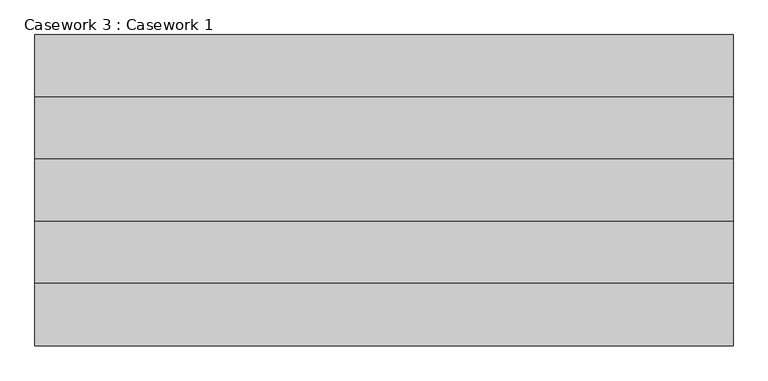
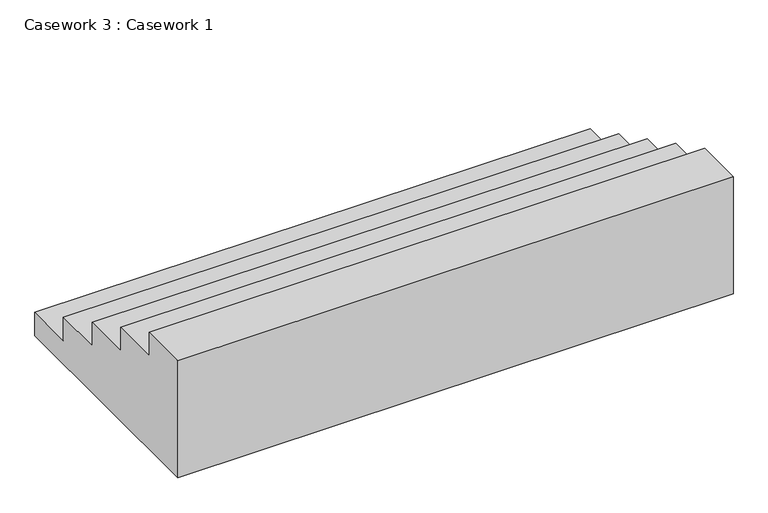
"""IFC4 building model written with IfcOpenShell, lengths in millimetres: furniture geometry, Casework 3 : Casework 1."""

from ifc_helpers import new_model, si_unit, frame, origin, place, context, project, spatial, polyline, outline, extrude, source, transform, mapped, element, save


def casework_3_casework_1_715d5e0d(model_context):
    return source(origin(), model_context, "Body", "SweptSolid", [
        extrude(outline(polyline([(14835.7086582, 762.0), (14835.7086582, 609.6), (15140.5086582, 609.6), (15140.5086582, 457.2), (15445.3086582, 457.2), (15445.3086582, 304.8), (15750.1086582, 304.8), (15750.1086582, 152.4), (16054.9086582, 152.4), (16054.9086582, 0.0), (14530.9086582, 0.0), (14530.9086582, 762.0), (14835.7086582, 762.0)])), frame((3122.729041, 0.0, 0.0), z_axis=(1.0, 0.0, 0.0), x_axis=(0.0, 1.0, 0.0)), (0.0, 0.0, 1.0), 3419.1487451),
    ])


if __name__ == "__main__":
    model = new_model("IFC4")
    model_context = context("Model", 3, world=origin())
    ifc_project = project(units=[si_unit("LENGTHUNIT", "METRE", prefix="MILLI")], contexts=[model_context])
    site = spatial("IfcSite", under=ifc_project)
    building = spatial("IfcBuilding", under=site)
    placement = place(None, origin())
    casework_3_casework_1_shape = casework_3_casework_1_715d5e0d(model_context)
    element("IfcFurniture", 1, ObjectType="Casework 3 : Casework 1", at=placement, inside=building, context=model_context, shape_type="MappedRepresentation", body=[
        mapped(casework_3_casework_1_shape, transform((0.0, 0.0, 0.0), x_axis=(1.0, 0.0, 0.0), y_axis=(0.0, 1.0, 0.0), z_axis=(0.0, 0.0, 1.0))),
    ])
    save(model, "model.ifc")

# Revit data of these elements
# Element 1 (IfcFurniture, "Casework 3 : Casework 1")
#   Materials on its faces: "Damp-proofing"
# Materials
#   "Damp-proofing": class "Generic", colour RGB 127 127 127, transparency 0, Description = "Damp-proofing", Cost = 0
